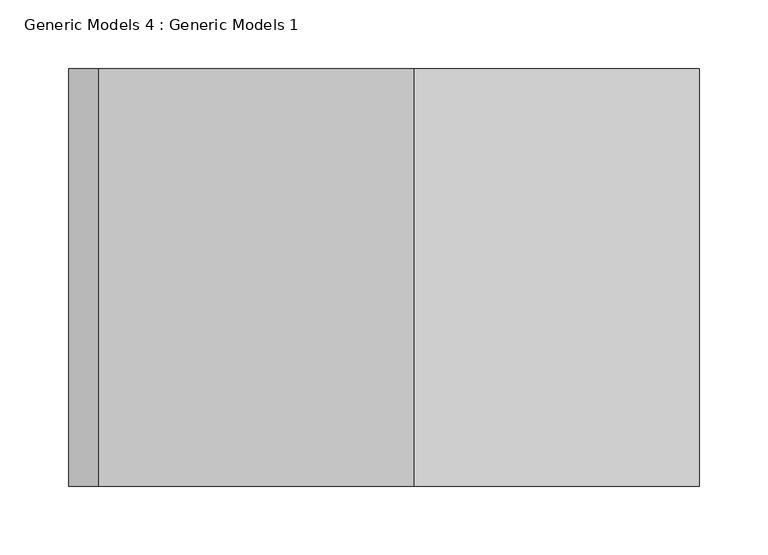
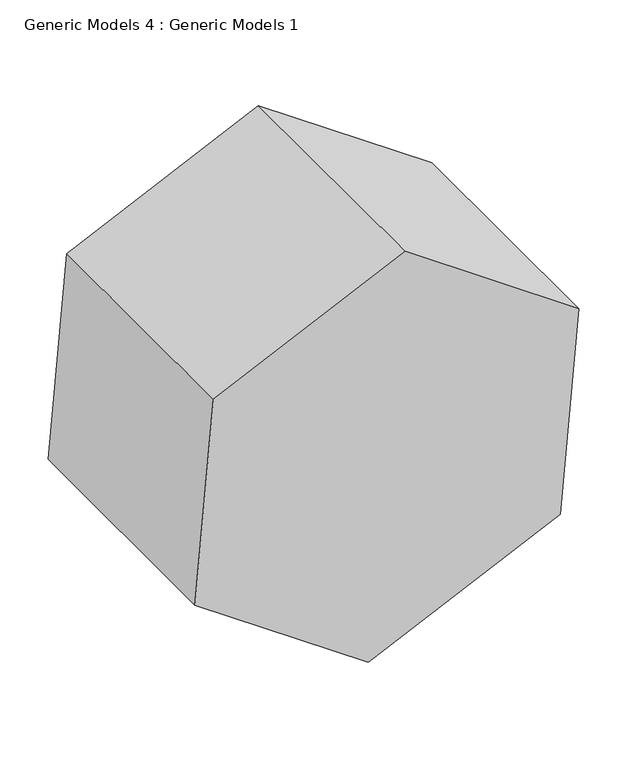
"""IFC4 building model written with IfcOpenShell, lengths in millimetres: proxy geometry, Generic Models 4 : Generic Models 1."""

from ifc_helpers import new_model, si_unit, frame, origin, place, context, project, spatial, polyline, outline, extrude, source, transform, mapped, element, save


def generic_models_4_generic_models_1_f88cb9c1(model_context):
    return source(origin(), model_context, "Body", "SweptSolid", [
        extrude(outline(polyline([(833.1013393, -4829.5079055), (978.7897542, -5037.5725247), (871.4447157, -5267.7747026), (618.4112624, -5289.9122613), (472.7228475, -5081.847642), (580.067886, -4851.6454641), (833.1013393, -4829.5079055)])), frame((0.0, -10720.3372434, 0.0), z_axis=(0.0, 1.0, 0.0), x_axis=(0.0, 0.0, 1.0)), (0.0, 0.0, 1.0), 304.8),
    ])


if __name__ == "__main__":
    model = new_model("IFC4")
    model_context = context("Model", 3, world=origin())
    ifc_project = project(units=[si_unit("LENGTHUNIT", "METRE", prefix="MILLI")], contexts=[model_context])
    site = spatial("IfcSite", under=ifc_project)
    building = spatial("IfcBuilding", under=site)
    placement = place(None, origin())
    generic_models_4_generic_models_1_shape = generic_models_4_generic_models_1_f88cb9c1(model_context)
    element("IfcBuildingElementProxy", 1, Name="Generic Models 4 : Generic Models 1", ObjectType="Generic Models 4 : Generic Models 1", at=placement, inside=building, context=model_context, shape_type="MappedRepresentation", body=[
        mapped(generic_models_4_generic_models_1_shape, transform((0.0, 0.0, 0.0), x_axis=(1.0, 0.0, 0.0), y_axis=(0.0, 1.0, 0.0), z_axis=(0.0, 0.0, 1.0))),
    ])
    save(model, "model.ifc")

# Revit data of these elements
# Element 1 (IfcBuildingElementProxy, "Generic Models 4 : Generic Models 1")
#   Materials on its faces: "Carpet (1)"
# Materials
#   "Carpet (1)": class "Carpet", colour RGB 124 80 67, transparency 0, Description = "Interior finish", Cost = 0
